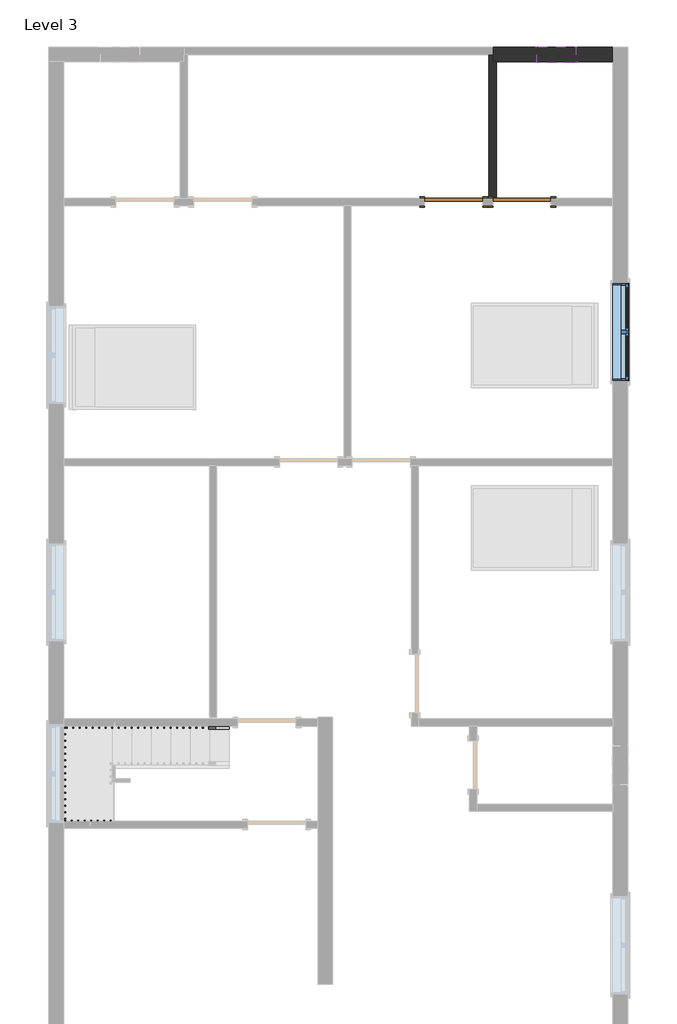
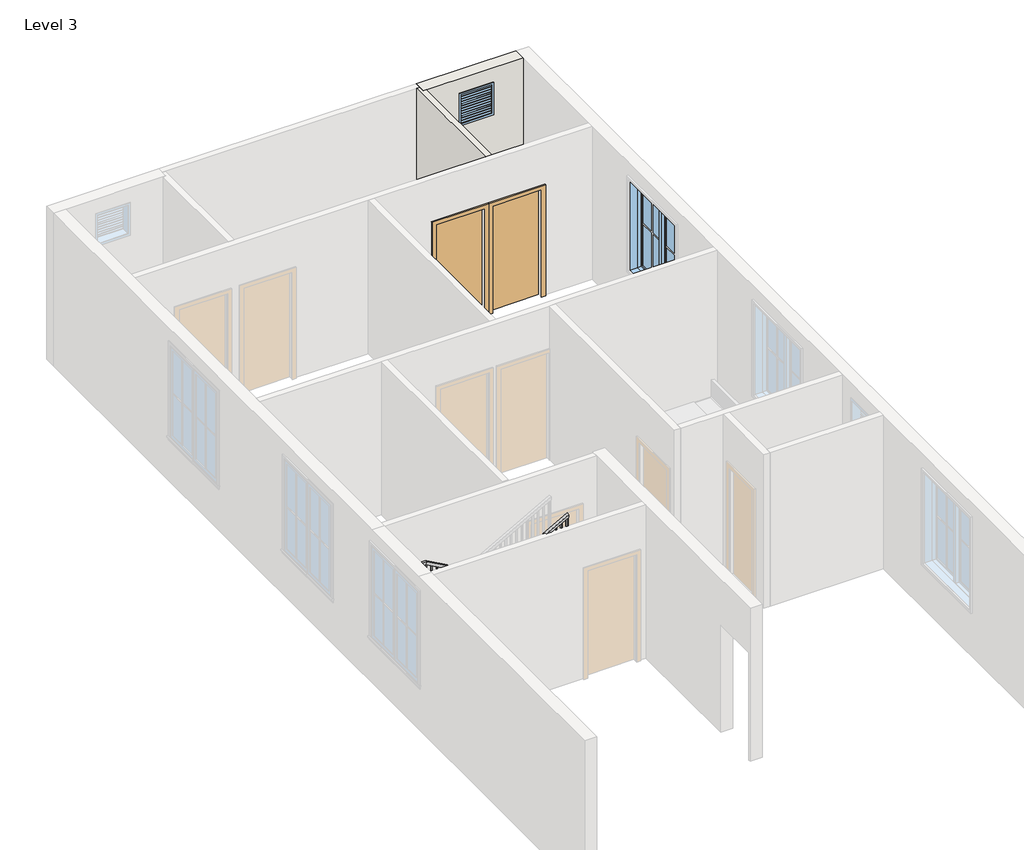
# One storey, part 2 of 3: 2 doors, 2 walls, 2 windows, 1 railing.
"""IFC4 building model written with IfcOpenShell, lengths in millimetres."""

from ifc_helpers import new_model, si_unit, frame, origin, place, context, project, spatial, polyline, outline, extrude, faceted_brep, transform, mapped, element, save
from components import single_flush_door_3_e5f9f3c4, single_flush_door_3_305aa2a5, window_casement_double_win_5_f93960c7, window_f2d8fef0

model = new_model("IFC4")

# Units and contexts
model_context = context("Model", 3, world=origin())
ifc_project = project(units=[si_unit("LENGTHUNIT", "METRE", prefix="MILLI")], contexts=[model_context])

# Site, building, storey
site = spatial("IfcSite", under=ifc_project)
building = spatial("IfcBuilding", under=site)
storey = spatial("IfcBuildingStorey", under=building, Name="Level 3", Elevation=3200.4)

# Doors
placement = place(None, origin())
single_flush_door_3_shape = single_flush_door_3_e5f9f3c4(model_context)
element("IfcDoor", 1, ObjectType="Single-Flush : DOOR 3'", at=placement, inside=storey, context=model_context, shape_type="MappedRepresentation", body=[
    mapped(single_flush_door_3_shape, transform((555.4379845, 6040.5434309, 3200.4), x_axis=(1.0, 0.0, 0.0), y_axis=(0.0, 1.0, 0.0), z_axis=(0.0, 0.0, 1.0))),
])
single_flush_door_3_2_shape = single_flush_door_3_305aa2a5(model_context)
element("IfcDoor", 2, ObjectType="Single-Flush : DOOR 3'", at=placement, inside=storey, context=model_context, shape_type="MappedRepresentation", body=[
    mapped(single_flush_door_3_2_shape, transform((1622.2379845, 6040.5434309, 3200.4), x_axis=(-1.0, 0.0, 0.0), y_axis=(0.0, -1.0, 0.0), z_axis=(0.0, 0.0, 1.0))),
])

# Railing
element("IfcRailing", 3, ObjectType="Handrail - Rectangular", at=placement, inside=storey, context=model_context, shape_type="SolidModel", body=[
    faceted_brep([(-2968.8120155, -2220.8065691, 4284.1333333), (-2968.8120155, -2220.8065691, 4226.020221), (-2968.8120155, -2170.0065691, 4226.020221), (-2968.8120155, -2170.0065691, 4284.1333333), (-4797.6120155, -2220.8065691, 5300.1333333), (-4810.7756177, -2220.8065691, 5249.3333333), (-4810.7756177, -2170.0065691, 5249.3333333), (-4797.6120155, -2170.0065691, 5300.1333333), (-5508.8120155, -2220.8065691, 5300.1333333), (-5508.8120155, -2220.8065691, 5249.3333333), (-5559.6120155, -2170.0065691, 5249.3333333), (-5559.6120155, -2170.0065691, 5300.1333333), (-5508.8120155, -3624.1565691, 5300.1333333), (-5508.8120155, -3624.1565691, 5249.3333333), (-5559.6120155, -3674.9565691, 5249.3333333), (-5559.6120155, -3674.9565691, 5300.1333333), (-5102.4120155, -3624.1565691, 5300.1333333), (-5089.2484132, -3624.1565691, 5249.3333333), (-5089.2484132, -3674.9565691, 5249.3333333), (-5102.4120155, -3674.9565691, 5300.1333333), (-2968.8120155, -3624.1565691, 6485.4666667), (-2968.8120155, -3674.9565691, 6485.4666667), (-2968.8120155, -3674.9565691, 6427.3535543), (-2968.8120155, -3624.1565691, 6427.3535543)], [[[0, 1, 2, 3]], [[1, 0, 4, 5]], [[2, 1, 5, 6]], [[3, 2, 6, 7]], [[0, 3, 7, 4]], [[5, 4, 8, 9]], [[6, 5, 9, 10]], [[7, 6, 10, 11]], [[4, 7, 11, 8]], [[9, 8, 12, 13]], [[10, 9, 13, 14]], [[11, 10, 14, 15]], [[8, 11, 15, 12]], [[13, 12, 16, 17]], [[14, 13, 17, 18]], [[15, 14, 18, 19]], [[12, 15, 19, 16]], [[20, 21, 22, 23]], [[17, 16, 20, 23]], [[18, 17, 23, 22]], [[19, 18, 22, 21]], [[16, 19, 21, 20]]]),
    extrude(outline(polyline([(6418.5341099, -2984.6870155), (6407.9507765, -3003.7370155), (5401.7333333, -3003.7370155), (5401.7333333, -2984.6870155), (6418.5341099, -2984.6870155)])), frame((0.0, -3659.0815691, 0.0), z_axis=(0.0, 1.0, 0.0), x_axis=(0.0, 0.0, 1.0)), (0.0, 0.0, 1.0), 19.05),
    extrude(outline(polyline([(6362.0896654, -3086.2870155), (6351.5063321, -3105.3370155), (5401.7333333, -3105.3370155), (5401.7333333, -3086.2870155), (6362.0896654, -3086.2870155)])), frame((0.0, -3659.0815691, 0.0), z_axis=(0.0, 1.0, 0.0), x_axis=(0.0, 0.0, 1.0)), (0.0, 0.0, 1.0), 19.05),
    extrude(outline(polyline([(6305.645221, -3187.8870155), (6295.0618876, -3206.9370155), (5401.7333333, -3206.9370155), (5401.7333333, -3187.8870155), (6305.645221, -3187.8870155)])), frame((0.0, -3659.0815691, 0.0), z_axis=(0.0, 1.0, 0.0), x_axis=(0.0, 0.0, 1.0)), (0.0, 0.0, 1.0), 19.05),
    extrude(outline(polyline([(6249.2007765, -3289.4870155), (6238.6174432, -3308.5370155), (5232.4, -3308.5370155), (5232.4, -3289.4870155), (6249.2007765, -3289.4870155)])), frame((0.0, -3659.0815691, 0.0), z_axis=(0.0, 1.0, 0.0), x_axis=(0.0, 0.0, 1.0)), (0.0, 0.0, 1.0), 19.05),
    extrude(outline(polyline([(6192.7563321, -3391.0870155), (6182.1729988, -3410.1370155), (5232.4, -3410.1370155), (5232.4, -3391.0870155), (6192.7563321, -3391.0870155)])), frame((0.0, -3659.0815691, 0.0), z_axis=(0.0, 1.0, 0.0), x_axis=(0.0, 0.0, 1.0)), (0.0, 0.0, 1.0), 19.05),
    extrude(outline(polyline([(6136.3118876, -3492.6870155), (6125.7285543, -3511.7370155), (5232.4, -3511.7370155), (5232.4, -3492.6870155), (6136.3118876, -3492.6870155)])), frame((0.0, -3659.0815691, 0.0), z_axis=(0.0, 1.0, 0.0), x_axis=(0.0, 0.0, 1.0)), (0.0, 0.0, 1.0), 19.05),
    extrude(outline(polyline([(6079.8674432, -3594.2870155), (6069.2841099, -3613.3370155), (5063.0666667, -3613.3370155), (5063.0666667, -3594.2870155), (6079.8674432, -3594.2870155)])), frame((0.0, -3659.0815691, 0.0), z_axis=(0.0, 1.0, 0.0), x_axis=(0.0, 0.0, 1.0)), (0.0, 0.0, 1.0), 19.05),
    extrude(outline(polyline([(6023.4229988, -3695.8870155), (6012.8396654, -3714.9370155), (5063.0666667, -3714.9370155), (5063.0666667, -3695.8870155), (6023.4229988, -3695.8870155)])), frame((0.0, -3659.0815691, 0.0), z_axis=(0.0, 1.0, 0.0), x_axis=(0.0, 0.0, 1.0)), (0.0, 0.0, 1.0), 19.05),
    extrude(outline(polyline([(5966.9785543, -3797.4870155), (5956.395221, -3816.5370155), (5063.0666667, -3816.5370155), (5063.0666667, -3797.4870155), (5966.9785543, -3797.4870155)])), frame((0.0, -3659.0815691, 0.0), z_axis=(0.0, 1.0, 0.0), x_axis=(0.0, 0.0, 1.0)), (0.0, 0.0, 1.0), 19.05),
    extrude(outline(polyline([(5910.5341099, -3899.0870155), (5899.9507765, -3918.1370155), (4893.7333333, -3918.1370155), (4893.7333333, -3899.0870155), (5910.5341099, -3899.0870155)])), frame((0.0, -3659.0815691, 0.0), z_axis=(0.0, 1.0, 0.0), x_axis=(0.0, 0.0, 1.0)), (0.0, 0.0, 1.0), 19.05),
    extrude(outline(polyline([(5854.0896654, -4000.6870155), (5843.5063321, -4019.7370155), (4893.7333333, -4019.7370155), (4893.7333333, -4000.6870155), (5854.0896654, -4000.6870155)])), frame((0.0, -3659.0815691, 0.0), z_axis=(0.0, 1.0, 0.0), x_axis=(0.0, 0.0, 1.0)), (0.0, 0.0, 1.0), 19.05),
    extrude(outline(polyline([(5797.645221, -4102.2870155), (5787.0618876, -4121.3370155), (4893.7333333, -4121.3370155), (4893.7333333, -4102.2870155), (5797.645221, -4102.2870155)])), frame((0.0, -3659.0815691, 0.0), z_axis=(0.0, 1.0, 0.0), x_axis=(0.0, 0.0, 1.0)), (0.0, 0.0, 1.0), 19.05),
    extrude(outline(polyline([(5741.2007765, -4203.8870155), (5730.6174432, -4222.9370155), (4724.4, -4222.9370155), (4724.4, -4203.8870155), (5741.2007765, -4203.8870155)])), frame((0.0, -3659.0815691, 0.0), z_axis=(0.0, 1.0, 0.0), x_axis=(0.0, 0.0, 1.0)), (0.0, 0.0, 1.0), 19.05),
    extrude(outline(polyline([(5684.7563321, -4305.4870155), (5674.1729988, -4324.5370155), (4724.4, -4324.5370155), (4724.4, -4305.4870155), (5684.7563321, -4305.4870155)])), frame((0.0, -3659.0815691, 0.0), z_axis=(0.0, 1.0, 0.0), x_axis=(0.0, 0.0, 1.0)), (0.0, 0.0, 1.0), 19.05),
    extrude(outline(polyline([(5628.3118876, -4407.0870155), (5617.7285543, -4426.1370155), (4724.4, -4426.1370155), (4724.4, -4407.0870155), (5628.3118876, -4407.0870155)])), frame((0.0, -3659.0815691, 0.0), z_axis=(0.0, 1.0, 0.0), x_axis=(0.0, 0.0, 1.0)), (0.0, 0.0, 1.0), 19.05),
    extrude(outline(polyline([(5571.8674432, -4508.6870155), (5561.2841099, -4527.7370155), (4555.0666667, -4527.7370155), (4555.0666667, -4508.6870155), (5571.8674432, -4508.6870155)])), frame((0.0, -3659.0815691, 0.0), z_axis=(0.0, 1.0, 0.0), x_axis=(0.0, 0.0, 1.0)), (0.0, 0.0, 1.0), 19.05),
    extrude(outline(polyline([(5515.4229988, -4610.2870155), (5504.8396654, -4629.3370155), (4555.0666667, -4629.3370155), (4555.0666667, -4610.2870155), (5515.4229988, -4610.2870155)])), frame((0.0, -3659.0815691, 0.0), z_axis=(0.0, 1.0, 0.0), x_axis=(0.0, 0.0, 1.0)), (0.0, 0.0, 1.0), 19.05),
    extrude(outline(polyline([(5458.9785543, -4711.8870155), (5448.395221, -4730.9370155), (4555.0666667, -4730.9370155), (4555.0666667, -4711.8870155), (5458.9785543, -4711.8870155)])), frame((0.0, -3659.0815691, 0.0), z_axis=(0.0, 1.0, 0.0), x_axis=(0.0, 0.0, 1.0)), (0.0, 0.0, 1.0), 19.05),
    extrude(outline(polyline([(5402.5341099, -4813.4870155), (5391.9507765, -4832.5370155), (4385.7333333, -4832.5370155), (4385.7333333, -4813.4870155), (5402.5341099, -4813.4870155)])), frame((0.0, -3659.0815691, 0.0), z_axis=(0.0, 1.0, 0.0), x_axis=(0.0, 0.0, 1.0)), (0.0, 0.0, 1.0), 19.05),
    extrude(outline(polyline([(5346.0896654, -4915.0870155), (5335.5063321, -4934.1370155), (4385.7333333, -4934.1370155), (4385.7333333, -4915.0870155), (5346.0896654, -4915.0870155)])), frame((0.0, -3659.0815691, 0.0), z_axis=(0.0, 1.0, 0.0), x_axis=(0.0, 0.0, 1.0)), (0.0, 0.0, 1.0), 19.05),
    extrude(outline(polyline([(5289.645221, -5016.6870155), (5279.0618876, -5035.7370155), (4385.7333333, -5035.7370155), (4385.7333333, -5016.6870155), (5289.645221, -5016.6870155)])), frame((0.0, -3659.0815691, 0.0), z_axis=(0.0, 1.0, 0.0), x_axis=(0.0, 0.0, 1.0)), (0.0, 0.0, 1.0), 19.05),
    extrude(outline(polyline([(-5137.3370155, -3659.0815691), (-5137.3370155, -3640.0315691), (-5118.2870155, -3640.0315691), (-5118.2870155, -3659.0815691), (-5137.3370155, -3659.0815691)])), frame((0.0, 0.0, 4385.7333333), z_axis=(0.0, 0.0, 1.0), x_axis=(1.0, 0.0, 0.0)), (0.0, 0.0, 1.0), 863.6),
    extrude(outline(polyline([(-5238.9370155, -3659.0815691), (-5238.9370155, -3640.0315691), (-5219.8870155, -3640.0315691), (-5219.8870155, -3659.0815691), (-5238.9370155, -3659.0815691)])), frame((0.0, 0.0, 4385.7333333), z_axis=(0.0, 0.0, 1.0), x_axis=(1.0, 0.0, 0.0)), (0.0, 0.0, 1.0), 863.6),
    extrude(outline(polyline([(-5340.5370155, -3659.0815691), (-5340.5370155, -3640.0315691), (-5321.4870155, -3640.0315691), (-5321.4870155, -3659.0815691), (-5340.5370155, -3659.0815691)])), frame((0.0, 0.0, 4385.7333333), z_axis=(0.0, 0.0, 1.0), x_axis=(1.0, 0.0, 0.0)), (0.0, 0.0, 1.0), 863.6),
    extrude(outline(polyline([(-5442.1370155, -3659.0815691), (-5442.1370155, -3640.0315691), (-5423.0870155, -3640.0315691), (-5423.0870155, -3659.0815691), (-5442.1370155, -3659.0815691)])), frame((0.0, 0.0, 4385.7333333), z_axis=(0.0, 0.0, 1.0), x_axis=(1.0, 0.0, 0.0)), (0.0, 0.0, 1.0), 863.6),
    extrude(outline(polyline([(-5543.7370155, -3608.2815691), (-5524.6870155, -3608.2815691), (-5524.6870155, -3627.3315691), (-5543.7370155, -3627.3315691), (-5543.7370155, -3608.2815691)])), frame((0.0, 0.0, 4385.7333333), z_axis=(0.0, 0.0, 1.0), x_axis=(1.0, 0.0, 0.0)), (0.0, 0.0, 1.0), 863.6),
    extrude(outline(polyline([(-5543.7370155, -3506.6815691), (-5524.6870155, -3506.6815691), (-5524.6870155, -3525.7315691), (-5543.7370155, -3525.7315691), (-5543.7370155, -3506.6815691)])), frame((0.0, 0.0, 4385.7333333), z_axis=(0.0, 0.0, 1.0), x_axis=(1.0, 0.0, 0.0)), (0.0, 0.0, 1.0), 863.6),
    extrude(outline(polyline([(-5543.7370155, -3405.0815691), (-5524.6870155, -3405.0815691), (-5524.6870155, -3424.1315691), (-5543.7370155, -3424.1315691), (-5543.7370155, -3405.0815691)])), frame((0.0, 0.0, 4385.7333333), z_axis=(0.0, 0.0, 1.0), x_axis=(1.0, 0.0, 0.0)), (0.0, 0.0, 1.0), 863.6),
    extrude(outline(polyline([(-5543.7370155, -3303.4815691), (-5524.6870155, -3303.4815691), (-5524.6870155, -3322.5315691), (-5543.7370155, -3322.5315691), (-5543.7370155, -3303.4815691)])), frame((0.0, 0.0, 4385.7333333), z_axis=(0.0, 0.0, 1.0), x_axis=(1.0, 0.0, 0.0)), (0.0, 0.0, 1.0), 863.6),
    extrude(outline(polyline([(-5543.7370155, -3201.8815691), (-5524.6870155, -3201.8815691), (-5524.6870155, -3220.9315691), (-5543.7370155, -3220.9315691), (-5543.7370155, -3201.8815691)])), frame((0.0, 0.0, 4385.7333333), z_axis=(0.0, 0.0, 1.0), x_axis=(1.0, 0.0, 0.0)), (0.0, 0.0, 1.0), 863.6),
    extrude(outline(polyline([(-5543.7370155, -3100.2815691), (-5524.6870155, -3100.2815691), (-5524.6870155, -3119.3315691), (-5543.7370155, -3119.3315691), (-5543.7370155, -3100.2815691)])), frame((0.0, 0.0, 4385.7333333), z_axis=(0.0, 0.0, 1.0), x_axis=(1.0, 0.0, 0.0)), (0.0, 0.0, 1.0), 863.6),
    extrude(outline(polyline([(-5543.7370155, -2998.6815691), (-5524.6870155, -2998.6815691), (-5524.6870155, -3017.7315691), (-5543.7370155, -3017.7315691), (-5543.7370155, -2998.6815691)])), frame((0.0, 0.0, 4385.7333333), z_axis=(0.0, 0.0, 1.0), x_axis=(1.0, 0.0, 0.0)), (0.0, 0.0, 1.0), 863.6),
    extrude(outline(polyline([(-5543.7370155, -2897.0815691), (-5524.6870155, -2897.0815691), (-5524.6870155, -2916.1315691), (-5543.7370155, -2916.1315691), (-5543.7370155, -2897.0815691)])), frame((0.0, 0.0, 4385.7333333), z_axis=(0.0, 0.0, 1.0), x_axis=(1.0, 0.0, 0.0)), (0.0, 0.0, 1.0), 863.6),
    extrude(outline(polyline([(-5543.7370155, -2795.4815691), (-5524.6870155, -2795.4815691), (-5524.6870155, -2814.5315691), (-5543.7370155, -2814.5315691), (-5543.7370155, -2795.4815691)])), frame((0.0, 0.0, 4385.7333333), z_axis=(0.0, 0.0, 1.0), x_axis=(1.0, 0.0, 0.0)), (0.0, 0.0, 1.0), 863.6),
    extrude(outline(polyline([(-5543.7370155, -2693.8815691), (-5524.6870155, -2693.8815691), (-5524.6870155, -2712.9315691), (-5543.7370155, -2712.9315691), (-5543.7370155, -2693.8815691)])), frame((0.0, 0.0, 4385.7333333), z_axis=(0.0, 0.0, 1.0), x_axis=(1.0, 0.0, 0.0)), (0.0, 0.0, 1.0), 863.6),
    extrude(outline(polyline([(-5543.7370155, -2592.2815691), (-5524.6870155, -2592.2815691), (-5524.6870155, -2611.3315691), (-5543.7370155, -2611.3315691), (-5543.7370155, -2592.2815691)])), frame((0.0, 0.0, 4385.7333333), z_axis=(0.0, 0.0, 1.0), x_axis=(1.0, 0.0, 0.0)), (0.0, 0.0, 1.0), 863.6),
    extrude(outline(polyline([(-5543.7370155, -2490.6815691), (-5524.6870155, -2490.6815691), (-5524.6870155, -2509.7315691), (-5543.7370155, -2509.7315691), (-5543.7370155, -2490.6815691)])), frame((0.0, 0.0, 4385.7333333), z_axis=(0.0, 0.0, 1.0), x_axis=(1.0, 0.0, 0.0)), (0.0, 0.0, 1.0), 863.6),
    extrude(outline(polyline([(-5543.7370155, -2389.0815691), (-5524.6870155, -2389.0815691), (-5524.6870155, -2408.1315691), (-5543.7370155, -2408.1315691), (-5543.7370155, -2389.0815691)])), frame((0.0, 0.0, 4385.7333333), z_axis=(0.0, 0.0, 1.0), x_axis=(1.0, 0.0, 0.0)), (0.0, 0.0, 1.0), 863.6),
    extrude(outline(polyline([(-5543.7370155, -2287.4815691), (-5524.6870155, -2287.4815691), (-5524.6870155, -2306.5315691), (-5543.7370155, -2306.5315691), (-5543.7370155, -2287.4815691)])), frame((0.0, 0.0, 4385.7333333), z_axis=(0.0, 0.0, 1.0), x_axis=(1.0, 0.0, 0.0)), (0.0, 0.0, 1.0), 863.6),
    extrude(outline(polyline([(-5499.2870155, -2185.8815691), (-5499.2870155, -2204.9315691), (-5518.3370155, -2204.9315691), (-5518.3370155, -2185.8815691), (-5499.2870155, -2185.8815691)])), frame((0.0, 0.0, 4385.7333333), z_axis=(0.0, 0.0, 1.0), x_axis=(1.0, 0.0, 0.0)), (0.0, 0.0, 1.0), 863.6),
    extrude(outline(polyline([(-5397.6870155, -2185.8815691), (-5397.6870155, -2204.9315691), (-5416.7370155, -2204.9315691), (-5416.7370155, -2185.8815691), (-5397.6870155, -2185.8815691)])), frame((0.0, 0.0, 4385.7333333), z_axis=(0.0, 0.0, 1.0), x_axis=(1.0, 0.0, 0.0)), (0.0, 0.0, 1.0), 863.6),
    extrude(outline(polyline([(-5296.0870155, -2185.8815691), (-5296.0870155, -2204.9315691), (-5315.1370155, -2204.9315691), (-5315.1370155, -2185.8815691), (-5296.0870155, -2185.8815691)])), frame((0.0, 0.0, 4385.7333333), z_axis=(0.0, 0.0, 1.0), x_axis=(1.0, 0.0, 0.0)), (0.0, 0.0, 1.0), 863.6),
    extrude(outline(polyline([(-5194.4870155, -2185.8815691), (-5194.4870155, -2204.9315691), (-5213.5370155, -2204.9315691), (-5213.5370155, -2185.8815691), (-5194.4870155, -2185.8815691)])), frame((0.0, 0.0, 4385.7333333), z_axis=(0.0, 0.0, 1.0), x_axis=(1.0, 0.0, 0.0)), (0.0, 0.0, 1.0), 863.6),
    extrude(outline(polyline([(-5092.8870155, -2185.8815691), (-5092.8870155, -2204.9315691), (-5111.9370155, -2204.9315691), (-5111.9370155, -2185.8815691), (-5092.8870155, -2185.8815691)])), frame((0.0, 0.0, 4385.7333333), z_axis=(0.0, 0.0, 1.0), x_axis=(1.0, 0.0, 0.0)), (0.0, 0.0, 1.0), 863.6),
    extrude(outline(polyline([(-4991.2870155, -2185.8815691), (-4991.2870155, -2204.9315691), (-5010.3370155, -2204.9315691), (-5010.3370155, -2185.8815691), (-4991.2870155, -2185.8815691)])), frame((0.0, 0.0, 4385.7333333), z_axis=(0.0, 0.0, 1.0), x_axis=(1.0, 0.0, 0.0)), (0.0, 0.0, 1.0), 863.6),
    extrude(outline(polyline([(-4889.6870155, -2185.8815691), (-4889.6870155, -2204.9315691), (-4908.7370155, -2204.9315691), (-4908.7370155, -2185.8815691), (-4889.6870155, -2185.8815691)])), frame((0.0, 0.0, 4385.7333333), z_axis=(0.0, 0.0, 1.0), x_axis=(1.0, 0.0, 0.0)), (0.0, 0.0, 1.0), 863.6),
    extrude(outline(polyline([(5236.7285543, -4788.0870155), (5247.3118876, -4807.1370155), (4385.7333333, -4807.1370155), (4385.7333333, -4788.0870155), (5236.7285543, -4788.0870155)])), frame((0.0, -2204.9315691, 0.0), z_axis=(0.0, 1.0, 0.0), x_axis=(0.0, 0.0, 1.0)), (0.0, 0.0, 1.0), 19.05),
    extrude(outline(polyline([(5180.2841099, -4686.4870155), (5190.8674432, -4705.5370155), (4216.4, -4705.5370155), (4216.4, -4686.4870155), (5180.2841099, -4686.4870155)])), frame((0.0, -2204.9315691, 0.0), z_axis=(0.0, 1.0, 0.0), x_axis=(0.0, 0.0, 1.0)), (0.0, 0.0, 1.0), 19.05),
    extrude(outline(polyline([(5123.8396654, -4584.8870155), (5134.4229988, -4603.9370155), (4216.4, -4603.9370155), (4216.4, -4584.8870155), (5123.8396654, -4584.8870155)])), frame((0.0, -2204.9315691, 0.0), z_axis=(0.0, 1.0, 0.0), x_axis=(0.0, 0.0, 1.0)), (0.0, 0.0, 1.0), 19.05),
    extrude(outline(polyline([(5067.395221, -4483.2870155), (5077.9785543, -4502.3370155), (4216.4, -4502.3370155), (4216.4, -4483.2870155), (5067.395221, -4483.2870155)])), frame((0.0, -2204.9315691, 0.0), z_axis=(0.0, 1.0, 0.0), x_axis=(0.0, 0.0, 1.0)), (0.0, 0.0, 1.0), 19.05),
    extrude(outline(polyline([(5010.9507765, -4381.6870155), (5021.5341099, -4400.7370155), (4047.0666667, -4400.7370155), (4047.0666667, -4381.6870155), (5010.9507765, -4381.6870155)])), frame((0.0, -2204.9315691, 0.0), z_axis=(0.0, 1.0, 0.0), x_axis=(0.0, 0.0, 1.0)), (0.0, 0.0, 1.0), 19.05),
    extrude(outline(polyline([(4954.5063321, -4280.0870155), (4965.0896654, -4299.1370155), (4047.0666667, -4299.1370155), (4047.0666667, -4280.0870155), (4954.5063321, -4280.0870155)])), frame((0.0, -2204.9315691, 0.0), z_axis=(0.0, 1.0, 0.0), x_axis=(0.0, 0.0, 1.0)), (0.0, 0.0, 1.0), 19.05),
    extrude(outline(polyline([(4898.0618876, -4178.4870155), (4908.645221, -4197.5370155), (4047.0666667, -4197.5370155), (4047.0666667, -4178.4870155), (4898.0618876, -4178.4870155)])), frame((0.0, -2204.9315691, 0.0), z_axis=(0.0, 1.0, 0.0), x_axis=(0.0, 0.0, 1.0)), (0.0, 0.0, 1.0), 19.05),
    extrude(outline(polyline([(4841.6174432, -4076.8870155), (4852.2007765, -4095.9370155), (3877.7333333, -4095.9370155), (3877.7333333, -4076.8870155), (4841.6174432, -4076.8870155)])), frame((0.0, -2204.9315691, 0.0), z_axis=(0.0, 1.0, 0.0), x_axis=(0.0, 0.0, 1.0)), (0.0, 0.0, 1.0), 19.05),
    extrude(outline(polyline([(4785.1729988, -3975.2870155), (4795.7563321, -3994.3370155), (3877.7333333, -3994.3370155), (3877.7333333, -3975.2870155), (4785.1729988, -3975.2870155)])), frame((0.0, -2204.9315691, 0.0), z_axis=(0.0, 1.0, 0.0), x_axis=(0.0, 0.0, 1.0)), (0.0, 0.0, 1.0), 19.05),
    extrude(outline(polyline([(4728.7285543, -3873.6870155), (4739.3118876, -3892.7370155), (3877.7333333, -3892.7370155), (3877.7333333, -3873.6870155), (4728.7285543, -3873.6870155)])), frame((0.0, -2204.9315691, 0.0), z_axis=(0.0, 1.0, 0.0), x_axis=(0.0, 0.0, 1.0)), (0.0, 0.0, 1.0), 19.05),
    extrude(outline(polyline([(4672.2841099, -3772.0870155), (4682.8674432, -3791.1370155), (3708.4, -3791.1370155), (3708.4, -3772.0870155), (4672.2841099, -3772.0870155)])), frame((0.0, -2204.9315691, 0.0), z_axis=(0.0, 1.0, 0.0), x_axis=(0.0, 0.0, 1.0)), (0.0, 0.0, 1.0), 19.05),
    extrude(outline(polyline([(4615.8396654, -3670.4870155), (4626.4229988, -3689.5370155), (3708.4, -3689.5370155), (3708.4, -3670.4870155), (4615.8396654, -3670.4870155)])), frame((0.0, -2204.9315691, 0.0), z_axis=(0.0, 1.0, 0.0), x_axis=(0.0, 0.0, 1.0)), (0.0, 0.0, 1.0), 19.05),
    extrude(outline(polyline([(4559.395221, -3568.8870155), (4569.9785543, -3587.9370155), (3708.4, -3587.9370155), (3708.4, -3568.8870155), (4559.395221, -3568.8870155)])), frame((0.0, -2204.9315691, 0.0), z_axis=(0.0, 1.0, 0.0), x_axis=(0.0, 0.0, 1.0)), (0.0, 0.0, 1.0), 19.05),
    extrude(outline(polyline([(4502.9507765, -3467.2870155), (4513.5341099, -3486.3370155), (3539.0666667, -3486.3370155), (3539.0666667, -3467.2870155), (4502.9507765, -3467.2870155)])), frame((0.0, -2204.9315691, 0.0), z_axis=(0.0, 1.0, 0.0), x_axis=(0.0, 0.0, 1.0)), (0.0, 0.0, 1.0), 19.05),
    extrude(outline(polyline([(4446.5063321, -3365.6870155), (4457.0896654, -3384.7370155), (3539.0666667, -3384.7370155), (3539.0666667, -3365.6870155), (4446.5063321, -3365.6870155)])), frame((0.0, -2204.9315691, 0.0), z_axis=(0.0, 1.0, 0.0), x_axis=(0.0, 0.0, 1.0)), (0.0, 0.0, 1.0), 19.05),
    extrude(outline(polyline([(4390.0618876, -3264.0870155), (4400.645221, -3283.1370155), (3539.0666667, -3283.1370155), (3539.0666667, -3264.0870155), (4390.0618876, -3264.0870155)])), frame((0.0, -2204.9315691, 0.0), z_axis=(0.0, 1.0, 0.0), x_axis=(0.0, 0.0, 1.0)), (0.0, 0.0, 1.0), 19.05),
    extrude(outline(polyline([(4333.6174432, -3162.4870155), (4344.2007765, -3181.5370155), (3369.7333333, -3181.5370155), (3369.7333333, -3162.4870155), (4333.6174432, -3162.4870155)])), frame((0.0, -2204.9315691, 0.0), z_axis=(0.0, 1.0, 0.0), x_axis=(0.0, 0.0, 1.0)), (0.0, 0.0, 1.0), 19.05),
    extrude(outline(polyline([(4277.1729988, -3060.8870155), (4287.7563321, -3079.9370155), (3369.7333333, -3079.9370155), (3369.7333333, -3060.8870155), (4277.1729988, -3060.8870155)])), frame((0.0, -2204.9315691, 0.0), z_axis=(0.0, 1.0, 0.0), x_axis=(0.0, 0.0, 1.0)), (0.0, 0.0, 1.0), 19.05),
    extrude(outline(polyline([(-5543.7370155, -3640.0315691), (-5524.6870155, -3640.0315691), (-5524.6870155, -3659.0815691), (-5543.7370155, -3659.0815691), (-5543.7370155, -3640.0315691)])), frame((0.0, 0.0, 4385.7333333), z_axis=(0.0, 0.0, 1.0), x_axis=(1.0, 0.0, 0.0)), (0.0, 0.0, 1.0), 863.6),
    extrude(outline(polyline([(-5524.6870155, -2185.8815691), (-5524.6870155, -2204.9315691), (-5543.7370155, -2204.9315691), (-5543.7370155, -2185.8815691), (-5524.6870155, -2185.8815691)])), frame((0.0, 0.0, 4385.7333333), z_axis=(0.0, 0.0, 1.0), x_axis=(1.0, 0.0, 0.0)), (0.0, 0.0, 1.0), 863.6),
    extrude(outline(polyline([(6427.3535543, -2968.8120155), (6416.770221, -2987.8620155), (5401.7333333, -2987.8620155), (5401.7333333, -2968.8120155), (6427.3535543, -2968.8120155)])), frame((0.0, -3659.0815691, 0.0), z_axis=(0.0, 1.0, 0.0), x_axis=(0.0, 0.0, 1.0)), (0.0, 0.0, 1.0), 19.05),
    extrude(outline(polyline([(4226.020221, -2968.8120155), (4236.6035543, -2987.8620155), (3369.7333333, -2987.8620155), (3369.7333333, -2968.8120155), (4226.020221, -2968.8120155)])), frame((0.0, -2204.9315691, 0.0), z_axis=(0.0, 1.0, 0.0), x_axis=(0.0, 0.0, 1.0)), (0.0, 0.0, 1.0), 19.05),
])

# Walls
element("IfcWall", 4, ObjectType="WALL 4.5\"", at=placement, inside=storey, context=model_context, shape_type="SweptSolid", body=[
    extrude(outline(polyline([(1107.8879845, 6097.6934309), (1107.8879845, 8345.5934309), (1165.0379845, 8345.5934309), (1165.0379845, 8231.2934309), (1222.1879845, 8231.2934309), (1222.1879845, 6097.6934309), (1107.8879845, 6097.6934309)])), frame((0.0, 0.0, 3200.4), z_axis=(0.0, 0.0, 1.0), x_axis=(1.0, 0.0, 0.0)), (0.0, 0.0, 1.0), 3048.0),
])
element("IfcWall", 5, ObjectType="WALL 9\"", at=placement, inside=storey, context=model_context, shape_type="Brep", body=[
    faceted_brep([(3050.9879845, 8459.8934309, 3200.4), (1165.0379845, 8459.8934309, 3200.4), (1165.0379845, 8459.8934309, 6248.4), (3050.9879845, 8459.8934309, 6248.4), (2469.9629845, 8459.8934309, 5943.6), (1860.3629845, 8459.8934309, 5943.6), (1860.3629845, 8459.8934309, 5334.0), (2469.9629845, 8459.8934309, 5334.0), (3050.9879845, 8231.2934309, 3200.4), (3050.9879845, 8231.2934309, 6248.4), (1222.1879845, 8231.2934309, 6248.4), (1165.0379845, 8231.2934309, 6248.4), (1165.0379845, 8231.2934309, 3200.4), (1222.1879845, 8231.2934309, 3200.4), (2469.9629845, 8231.2934309, 5943.6), (2469.9629845, 8231.2934309, 5334.0), (1860.3629845, 8231.2934309, 5334.0), (1860.3629845, 8231.2934309, 5943.6), (1165.0379845, 8345.5934309, 3200.4), (1165.0379845, 8345.5934309, 6248.4)], [[[0, 1, 2, 3], [4, 5, 6, 7]], [[8, 9, 10, 11, 12, 13], [14, 15, 16, 17]], [[1, 0, 8, 13, 12, 18]], [[2, 1, 18, 12, 11, 19]], [[0, 3, 9, 8]], [[15, 14, 4, 7]], [[16, 15, 7, 6]], [[17, 16, 6, 5]], [[14, 17, 5, 4]], [[3, 2, 19, 11, 10, 9]]]),
])

# Windows
window_casement_double_win_5_shape = window_casement_double_win_5_f93960c7(model_context)
element("IfcWindow", 6, ObjectType="Window-Casement-Double : WIN 5'", at=placement, inside=storey, context=model_context, shape_type="MappedRepresentation", body=[
    mapped(window_casement_double_win_5_shape, transform((3165.2879845, 4002.1934309, 3200.4), x_axis=(0.0, -1.0, 0.0), y_axis=(1.0, 0.0, 0.0), z_axis=(0.0, 0.0, 1.0))),
])
window_shape = window_f2d8fef0(model_context)
element("IfcWindow", 7, ObjectType="Window-Louvers : 24\" x 24\"", at=placement, inside=storey, context=model_context, shape_type="MappedRepresentation", body=[
    mapped(window_shape, transform((2165.1629845, 8339.2434309, 4419.6), x_axis=(-1.0, 0.0, 0.0), y_axis=(0.0, -1.0, 0.0), z_axis=(0.0, 0.0, 1.0))),
])

save(model, "model.ifc")

# Revit data of these elements
# Type "Single-Flush : DOOR 3'"
#   Type Mark = "9"
#   Construction Type Id = "MDOOR"
#   Assembly Code = "C1020"
#   Analytic Construction = "Metal"
#   Thickness = 0' - 2"
#   Heat Transfer Coefficient (U) = 0.651978 BTU/(h·ft²·°F)
#   Height = 7' - 0"
#   Trim Projection Ext = 0' - 1"
#   Trim Projection Int = 0' - 1"
#   Trim Width = 0' - 3"
#   Width = 3' - 0"
#   Define Thermal Properties by = 1
#   Door Material = Door - Panel
#   Frame Material = Door - Frame
#   Visual Light Transmittance = 0
#   Solar Heat Gain Coefficient = 0
#   Function = (empty or 0)
#   Wall Closure = (empty or 0)
# Type "Handrail - Rectangular"
#   Assembly Code = "C2010400"
#   built-in parameter 1008612 = 0.0416667 (stored number, unit not read)
#   built-in parameter 1008611 = 0.0416667 (stored number, unit not read)
#   built-in parameter 1008609 = 0.333333 (stored number, unit not read)
#   built-in parameter 1008604 = 0.166667 (stored number, unit not read)
#   built-in parameter 1008603 = 0.166667 (stored number, unit not read)
#   Railing Height = 3' - 0"
#   built-in parameter 1008630 = 2
#   built-in parameter 1008610 = 2
#   built-in parameter 1008618 = Baluster - Square : 3/4"
# Type "WALL 4.5\""
#   Assembly Code = "B2010"
#   Layers, outside or top first: 0' - 4 1/2" no material (function 1)
# Type "WALL 9\""
#   Assembly Code = "B2010"
#   Layers, outside or top first: 0' - 9" no material (function 1)
# Type "Window-Casement-Double : WIN 5'"
#   Type Mark = "18"
#   Fire Rating = "0.5h"
#   Assembly Code = "B2020100"
#   Analytic Construction = "Double glazing - domestic"
#   Frame Extension [instance default] = 0' - 0 1/4"
#   Window Inset [instance default] = 0' - 0"
#   Wall Thickness [instance default] = 0' - 6"
#   Interior Wall Closure [instance default] = 0' - 2 1/4"
#   Half Width = 2' - 6"
#   Visual Light Transmittance = 0.81
#   Thermal Resistance (R) = 1.8146 (h·ft²·°F)/BTU
#   Solar Heat Gain Coefficient = 0.76
#   Rough Width = 5' - 0 1/2"
#   Rough Height = 6' - 0 1/2"
#   Height = 6' - 0"
#   Heat Transfer Coefficient (U) = 0.5511 BTU/(h·ft²·°F)
#   Exterior Wall Closure [instance default] = 0' - 1 1/4"
#   Extension Jamb [instance default] = 0' - 2 1/4"
#   Default Sill Height = 3' - 0"
#   Width = 5' - 0"
#   Muntin Visibility = yes
#   Interior Trim Visibility [instance default] = yes
#   Exterior Trim Visibility [instance default] = yes
#   Extension Jamb Visibility [instance default] = yes
#   Interior Trim Material = Wood - Stained
#   Muntin Pattern = Muntin Pattern_2x2 : Muntin Pattern_2x2
#   Interior Trim = Trim-Window-Interior-Flat : Picture Frame
#   Interior Frame Material = Wood - Stained
#   Glass Panel Material = Glass
#   Exterior Trim Material = Clad - White
#   Exterior Trim = Trim-Window-Exterior-Flat : with Sill
#   Exterior Frame Material = Clad - White
#   Wall Closure = (empty or 0)
# Type "Window-Louvers : 24\" x 24\""
#   Type Mark = "19"
#   Construction Type Id = "GSP4R"
#   Assembly Code = "B20"
#   Analytic Construction = "1/8 in Pilkington single glazing"
#   Visual Light Transmittance = 0.9
#   Thermal Resistance (R) = 1.53941 (h·ft²·°F)/BTU
#   Solar Heat Gain Coefficient = 0.78
#   Max Height = 1' - 11.74264"
#   Height = 2' - 0"
#   Heat Transfer Coefficient (U) = 0.6496 BTU/(h·ft²·°F)
#   Blade Width [instance default] = 1' - 10 1/2"
#   Blade Vertical Thickness = 0' - 0.35355"
#   Blade Thickness = 0' - 0 1/4"
#   Blade Spacing = 0' - 1 1/2"
#   Blade Height = 0' - 1.85355"
#   Blade Depth = 0' - 3"
#   Blade Angle = 45.00°
#   Default Sill Height = 3' - 0"
#   Trim Projection_Exterior = 0' - 0 1/2"
#   Trim Projection_Interior = 0' - 0 1/2"
#   Trim Width_Exterior = 0' - 1 1/2"
#   Trim Width_Interior = 0' - 1 1/2"
#   Width = 2' - 0"
#   Max Blade Count = 12
#   Define Thermal Properties by = 1
#   Blade Count = 12
#   Frame Material = Birch
#   Louver Material = Birch
#   Trim Exterior Material = Birch
#   Trim Interior Material = Birch
#   Wall Closure = (empty or 0)
# Elements 1, 2 (IfcDoor, "Single-Flush : DOOR 3'")
#   Phase Created = New Construction
#   Materials on its faces: "Door - Frame", "Door - Panel"
# Element 3 (IfcRailing, "Handrail - Rectangular")
#   Phase Created = New Construction
# Element 4 (IfcWall, "WALL 4.5\"")
#   Top Offset = 0' - 0"
#   Base Offset = 0' - 0"
#   Unconnected Height = 10' - 0"
#   wall height = 10' - 0"
#   Phase Created = New Construction
#   Base Constraint = Level 3
#   Materials on its faces: "Default Wall"
# Element 5 (IfcWall, "WALL 9\"")
#   Top Offset = 0' - 0"
#   Base Offset = 0' - 0"
#   Unconnected Height = 10' - 0"
#   wall height = 10' - 0"
#   Phase Created = New Construction
#   Base Constraint = Level 3
#   Materials on its faces: "Default Wall", "Brick, Common"
# Element 6 (IfcWindow, "Window-Casement-Double : WIN 5'")
#   Mark = "12"
#   Window Inset = 0' - 0"
#   Interior Wall Closure = 0' - 2 1/4"
#   Frame Extension = 0' - 0 1/4"
#   Exterior Wall Closure = 0' - 1 1/4"
#   Interior Trim Visibility = yes
#   Exterior Trim Visibility = yes
#   Phase Created = New Construction
#   Materials on its faces: "Wood - Stained", "Glass", "Clad - White"
# Element 7 (IfcWindow, "Window-Louvers : 24\" x 24\"")
#   Mark = "19"
#   Blade Width = 1' - 10 1/2"
#   Phase Created = New Construction
#   Materials on its faces: "Birch"
# Materials
#   "Door - Panel": class "Wood", colour RGB 210 159 95, transparency 0, Cost = 0
#   "Door - Frame": colour RGB 118 70 51, transparency 0, Cost = 0
#   "Wood - Stained": class "Wood", colour RGB 224 178 126, transparency 0, Cost = 0
#   "Glass": class "Glass", colour RGB 0 128 192, transparency 0.75, Description = "Soda Lime Glass", Cost = 0
#   "Clad - White": class "Wood", colour RGB 242 242 238, transparency 0, Cost = 0
#   "Birch": class "Wood", colour RGB 224 178 126, transparency 0, Description = "Betula Alleghaniensis", Cost = 0
#   "Default Wall": colour RGB 128 128 128, transparency 0, Cost = 0
#   "Brick, Common": class "Masonry", colour RGB 170 98 104, transparency 0, Description = "Common brick", Cost = 0
